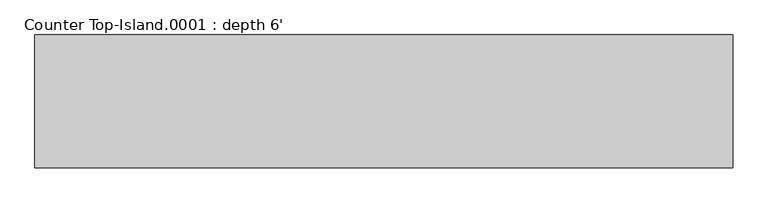
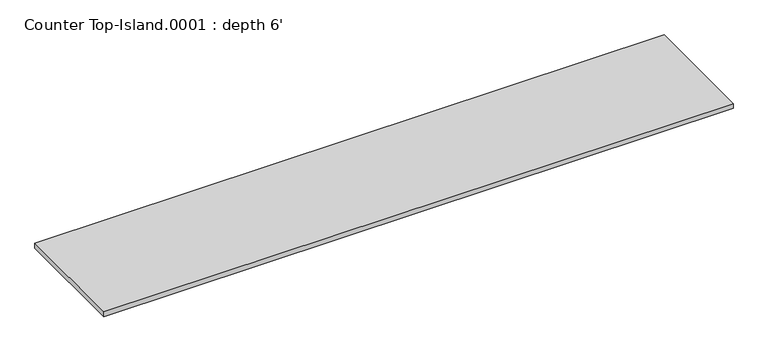
"""IFC4 building model written with IfcOpenShell, lengths in millimetres: furniture geometry, Counter Top-Island.0001 : depth 6'."""

from ifc_helpers import new_model, si_unit, frame, origin, place, context, project, spatial, polyline, outline, extrude, source, transform, mapped, element, save


def counter_top_island_0001_depth_6_5a0cf1da(model_context):
    return source(origin(), model_context, "Body", "SweptSolid", [
        extrude(outline(polyline([(3473.1377049, -25.4), (-1200.4622951, -25.4), (-1200.4622951, 863.6), (3473.1377049, 863.6), (3473.1377049, -25.4)])), frame((0.0, 0.0, 571.5), z_axis=(0.0, 0.0, 1.0), x_axis=(1.0, 0.0, 0.0)), (0.0, 0.0, 1.0), 38.1),
    ])


if __name__ == "__main__":
    model = new_model("IFC4")
    model_context = context("Model", 3, world=origin())
    ifc_project = project(units=[si_unit("LENGTHUNIT", "METRE", prefix="MILLI")], contexts=[model_context])
    site = spatial("IfcSite", under=ifc_project)
    building = spatial("IfcBuilding", under=site)
    placement = place(None, origin())
    counter_top_island_0001_depth_6_shape = counter_top_island_0001_depth_6_5a0cf1da(model_context)
    element("IfcFurniture", 1, ObjectType="Counter Top-Island.0001 : depth 6'", at=placement, inside=building, context=model_context, shape_type="MappedRepresentation", body=[
        mapped(counter_top_island_0001_depth_6_shape, transform((0.0, 0.0, 0.0), x_axis=(1.0, 0.0, 0.0), y_axis=(0.0, 1.0, 0.0), z_axis=(0.0, 0.0, 1.0))),
    ])
    save(model, "model.ifc")

# Revit data of these elements
# Type "Counter Top-Island.0001 : depth 6'"
#   Assembly Code = "C1030400"
#   Counter Thickness = 0' - 1 1/2"
#   Depth [instance default] = 4' - 2"
#   Height = 2' - 0"
#   Length [instance default] = 8' - 0"
#   Counter Top Material = none
#   Default Elevation = 0
# Element 1 (IfcFurniture, "Counter Top-Island.0001 : depth 6'")
#   Depth = 2' - 11"
#   Length = 15' - 4"
#   Materials on its faces: "Counter Top"
# Materials
#   "Counter Top": class "Wood", colour RGB 226 177 128, transparency 0
